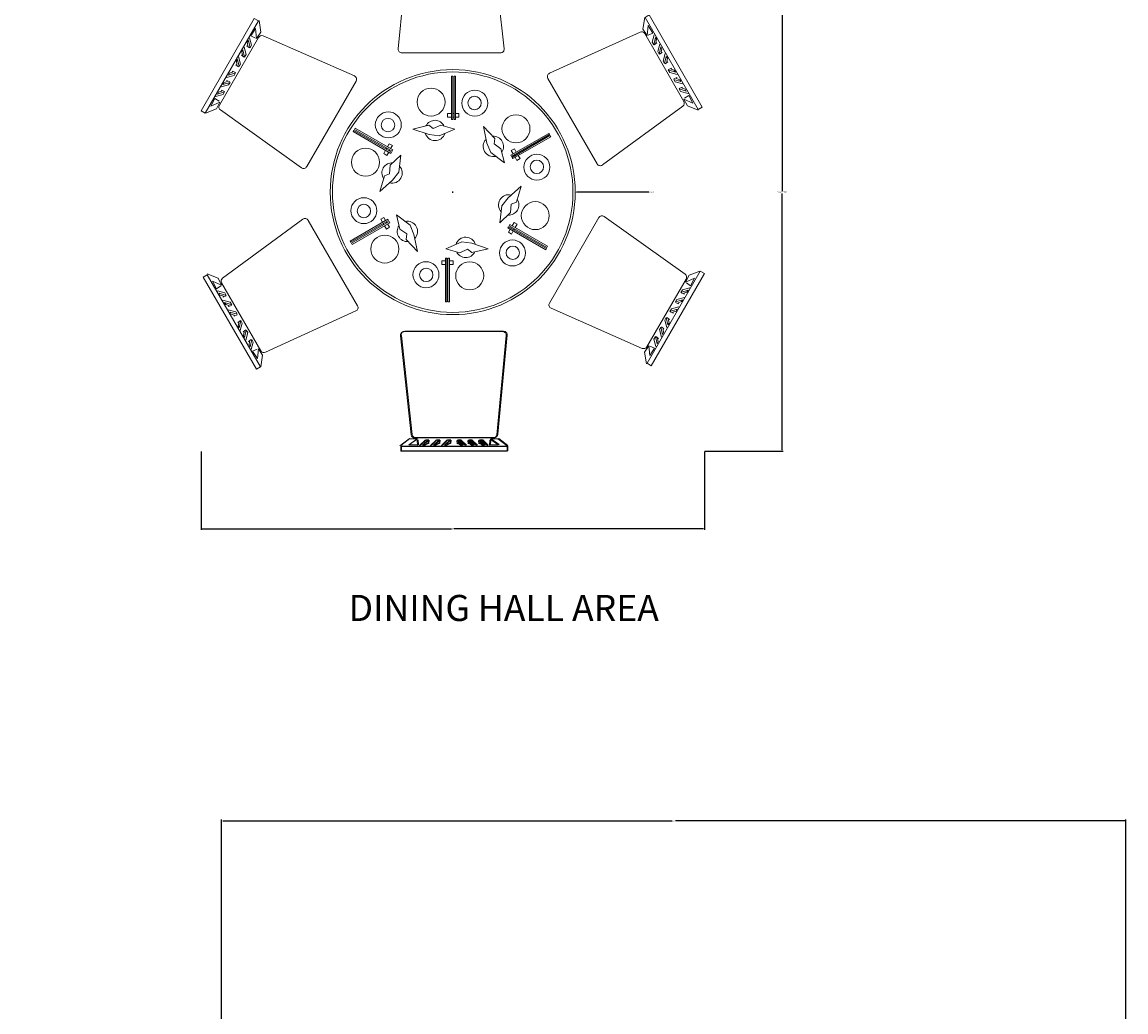
# Model space of a CAD drawing. Units: inches. Extents: x 1865 to 2541, y 1997 to 2759.
# Tile 4 of 11: x 2155 to 2346, y 2234 to 2405. Entities that reach past the tile are written whole.
import ezdxf

# ---------------------------------------------------------------- set-up
doc = ezdxf.new("R2010")
doc.units = ezdxf.units.IN
for name, color, linetype, lineweight in [('A-ANNO-DIMS', 2, 'Continuous', 18), ('A-AREA-IDEN', 4, 'Continuous', 18), ('DINING TABLE', 120, 'Continuous', 13)]:
    doc.layers.add(name, color=color, linetype=linetype, lineweight=lineweight)
doc.styles.get("Standard").update_dxf_attribs({"font": 'arial.ttf'})
doc.dimstyles.get("Standard").update_dxf_attribs({"dimtxt": 0.18, "dimasz": 0.18, "dimexe": 0.18, "dimexo": 0.0625, "dimgap": 0.09, "dimtad": 0, "dimtih": 1, "dimtoh": 1, "dimdec": 4, "dimzin": 0, "dimdsep": 46, "dimtxsty": 'Standard', "dimcen": 0.09, "dimadec": 0, "dimazin": 0, "dimtfac": 1, "dimtdec": 4, "dimtofl": 0, "dimtmove": 0, "dimatfit": 3, "dimfxl": 1, "dimtolj": 1, "dimtzin": 0, "dimarcsym": 0})

# ---------------------------------------------------------------- blocks, each defined once
blk = doc.blocks.new('A$C45501D90')
for p, q in [((-242.2, 1133.5), (224, 1133.5)), ((-242.2, 1112.8), (-242.2, 1133.5)), ((224, 1112.8), (-242.2, 1112.8)), ((224, 1112.8), (187.3, 1079.2)), ((224, 1133.5), (224, 1112.8)), ((-242.2, 1111.2), (-202.3, 1079.2)), ((-203.9, 1106.4), (-165.6, 1108)), ((-168.8, 1080.8), (-203.9, 1106.4)), ((-202.3, 1079.2), (-168.8, 1080.8)), ((161.8, 1076.1), (-181.4, 1076.1)), ((-165.6, 1108), (-167.2, 1085.6)), ((-156, 1109.6), (-132, 1085.6)), ((-119.3, 1085.6), (-143.2, 1108)), ((-143.2, 1108), (-133.6, 1108)), ((-133.6, 1108), (-122.5, 1098.4)), ((-132, 1085.6), (-119.3, 1085.6)), ((-122.5, 1098.4), (-119.3, 1101.6)), ((-119.3, 1101.6), (-117.7, 1087.2)), ((-108.1, 1109.6), (-84.1, 1085.6)), ((-71.4, 1085.6), (-95.3, 1108)), ((-95.3, 1108), (-85.7, 1108)), ((-85.7, 1108), (-74.6, 1098.4)), ((-84.1, 1085.6), (-71.4, 1085.6)), ((-74.6, 1098.4), (-71.4, 1101.6)), ((-71.4, 1101.6), (-69.8, 1087.2)), ((-60.2, 1109.6), (-36.2, 1085.6)), ((-23.5, 1085.6), (-47.4, 1108)), ((-47.4, 1108), (-37.8, 1108)), ((-37.8, 1108), (-26.7, 1098.4)), ((-36.2, 1085.6), (-23.5, 1085.6)), ((-26.7, 1098.4), (-23.5, 1101.6)), ((-23.5, 1101.6), (-21.9, 1087.2)), ((8.5, 1101.6), (6.9, 1087.2)), ((8.5, 1085.6), (32.4, 1108)), ((11.6, 1098.4), (8.5, 1101.6)), ((21.2, 1085.6), (8.5, 1085.6)), ((22.8, 1108), (11.6, 1098.4)), ((45.2, 1109.6), (21.2, 1085.6)), ((32.4, 1108), (22.8, 1108)), ((56.3, 1101.6), (54.8, 1087.2)), ((56.3, 1085.6), (80.3, 1108)), ((59.5, 1098.4), (56.3, 1101.6)), ((69.1, 1085.6), (56.3, 1085.6)), ((70.7, 1108), (59.5, 1098.4)), ((93.1, 1109.6), (69.1, 1085.6)), ((80.3, 1108), (70.7, 1108)), ((104.2, 1101.6), (102.6, 1087.2)), ((104.2, 1085.6), (128.2, 1108)), ((107.4, 1098.4), (104.2, 1101.6)), ((117, 1085.6), (104.2, 1085.6)), ((118.6, 1108), (107.4, 1098.4)), ((141, 1109.6), (117, 1085.6)), ((128.2, 1108), (118.6, 1108)), ((188.9, 1106.4), (150.5, 1108)), ((150.5, 1108), (152.1, 1085.6)), ((153.7, 1080.8), (188.9, 1106.4)), ((187.3, 1079.2), (153.7, 1080.8)), ((-197.3, 1061.6), (-238.9, 627.6)), ((225.2, 627.8), (177.6, 1061.8)), ((842.6, 766.1), (860.5, 776.5)), ((860.5, 776.5), (1093.6, 372.8)), ((-1102.7, 357), (-869.7, 760.7)), ((-851.7, 750.4), (-1084.8, 346.6)), ((-869.7, 760.7), (-851.7, 750.4)), ((-848.7, 752.3), (-841, 701.8)), ((841.2, 765.3), (833.5, 714.8)), ((1075.7, 362.4), (842.6, 766.1)), ((851.7, 686.6), (856.2, 729.8)), ((856.2, 729.8), (876.7, 697.4)), ((-851, 678.1), (-1022.6, 380.9)), ((-863.7, 716.7), (-884.3, 684.4)), ((-884.3, 684.4), (-864.1, 674.6)), ((-859.2, 673.6), (-863.7, 716.7)), ((-841, 701.8), (-859.2, 673.6)), ((-431.1, 509), (-830.8, 684.8)), ((820.7, 701.7), (424.1, 520.7)), ((833.5, 714.8), (851.7, 686.6)), ((1012.8, 397.9), (841.2, 695.1)), ((876.7, 697.4), (856.6, 687.6)), ((882.9, 689.9), (874.2, 657.2)), ((880.6, 646.1), (887.9, 678)), ((887.9, 678), (892.7, 669.7)), ((-914.4, 635.4), (-905.6, 602.7)), ((-897.5, 642.2), (-901.9, 641.1)), ((-901.9, 641.1), (-890.2, 632.5)), ((-895.4, 665), (-900.2, 656.7)), ((-900.2, 656.7), (-897.5, 642.2)), ((-888.1, 633.1), (-895.4, 665)), ((-890.4, 676.9), (-881.7, 644.2)), ((-881.7, 644.2), (-888.1, 633.1)), ((874.2, 657.2), (880.6, 646.1)), ((894.4, 654.1), (882.7, 645.5)), ((892.7, 669.7), (890, 655.2)), ((890, 655.2), (894.4, 654.1)), ((906.9, 648.4), (898.1, 615.7)), ((904.5, 604.6), (911.9, 636.5)), ((911.9, 636.5), (916.7, 628.2)), ((-943.3, 582), (-948.1, 573.8)), ((-936, 550.1), (-943.3, 582)), ((-938.3, 593.9), (-929.6, 561.2)), ((-921.5, 600.8), (-925.8, 599.6)), ((-925.8, 599.6), (-914.2, 591)), ((-919.4, 623.5), (-924.2, 615.2)), ((-924.2, 615.2), (-921.5, 600.8)), ((-912, 591.6), (-919.4, 623.5)), ((-905.6, 602.7), (-912, 591.6)), ((-223, 610.1), (209.4, 610.1)), ((898.1, 615.7), (904.5, 604.6)), ((918.3, 612.6), (906.7, 604)), ((916.7, 628.2), (914, 613.8)), ((914, 613.8), (918.3, 612.6)), ((930.8, 606.9), (922.1, 574.2)), ((928.4, 563.1), (935.8, 595.1)), ((935.8, 595.1), (940.6, 586.8)), ((940.6, 586.8), (937.9, 572.3)), ((-945.4, 559.3), (-949.8, 558.1)), ((-949.8, 558.1), (-938.1, 549.6)), ((-948.1, 573.8), (-945.4, 559.3)), ((-929.6, 561.2), (-936, 550.1)), ((922.1, 574.2), (928.4, 563.1)), ((942.3, 571.1), (930.6, 562.6)), ((937.9, 572.3), (942.3, 571.1)), ((950.8, 524.4), (944.4, 535.5)), ((944.4, 535.5), (975.7, 525.9)), ((958.2, 543.5), (945, 537.7)), ((957.1, 539.1), (958.2, 543.5)), ((970.9, 534.2), (957.1, 539.1)), ((975.7, 525.9), (970.9, 534.2)), ((-1002.4, 479.7), (-988.5, 484.6)), ((-991, 502.7), (-958.3, 511.4)), ((-988.5, 484.6), (-989.7, 489)), ((-989.7, 489), (-976.5, 483.2)), ((-951.9, 522.5), (-983.2, 512.9)), ((-983.2, 512.9), (-978.5, 521.2)), ((-978.5, 521.2), (-964.6, 526.1)), ((-964.6, 526.1), (-965.7, 530.5)), ((-965.7, 530.5), (-952.5, 524.7)), ((-958.3, 511.4), (-951.9, 522.5)), ((-639.9, 111.9), (-423.7, 486.4)), ((-5.6, 508.7, 90.8), (0.4, 508.7, 90.8)), ((-5.6, 317.7, 90.8), (-5.6, 508.7, 90.8)), ((0.4, 508.7, 90.8), (0.4, 317.7, 90.8)), ((5.8, 317.7, 90.8), (5.8, 508.7, 90.8)), ((5.8, 508.7, 90.8), (11.8, 508.7, 90.8)), ((11.8, 508.7, 90.8), (11.8, 317.7, 90.8)), ((416.9, 498.2), (633.1, 123.7)), ((983.5, 515.7), (950.8, 524.4)), ((968.4, 494), (999.7, 484.4)), ((974.7, 483), (968.4, 494)), ((982.2, 502), (968.9, 496.2)), ((981, 497.6), (982.2, 502)), ((994.9, 492.7), (981, 497.6)), ((999.7, 484.4), (994.9, 492.7)), ((-999.8, 439.5), (-1031.1, 430)), ((-1031.1, 430), (-1026.3, 438.3)), ((-1026.3, 438.3), (-1012.5, 443.1)), ((-1015, 461.2), (-982.3, 469.9)), ((-1012.5, 443.1), (-1013.6, 447.5)), ((-1013.6, 447.5), (-1000.4, 441.7)), ((-975.9, 481), (-1007.2, 471.4)), ((-1007.2, 471.4), (-1002.4, 479.7)), ((-1006.2, 428.5), (-999.8, 439.5)), ((-982.3, 469.9), (-975.9, 481)), ((1007.4, 474.2), (974.7, 483)), ((998.7, 441.5), (992.3, 452.5)), ((992.3, 452.5), (1023.6, 443)), ((1006.1, 460.5), (992.9, 454.7)), ((1031.4, 432.7), (998.7, 441.5)), ((1005, 456.2), (1006.1, 460.5)), ((1018.8, 451.3), (1005, 456.2)), ((1023.6, 443), (1018.8, 451.3)), ((-1060.1, 376.6), (-1042.3, 410.6)), ((-1020.4, 394.3), (-1060.1, 376.6)), ((-1042.3, 410.6), (-1023.8, 398.1)), ((-1038.9, 419.7), (-1006.2, 428.5)), ((-1035.8, 364.4), (-1020.4, 394.3)), ((1028.3, 377.5), (1012.9, 407.3)), ((1012.9, 407.3), (1052.6, 389.6)), ((1034.8, 423.6), (1016.3, 411.1)), ((1052.6, 389.6), (1034.8, 423.6)), ((-1084.8, 346.6), (-1102.7, 357)), ((-1083.4, 345.8), (-1035.8, 364.4)), ((-1018, 360), (-663, 106.9)), ((-22.3, 329.1, 90.8), (-22.3, 344.6, 90.8)), ((-22.3, 344.6, 90.8), (-5.6, 344.6, 90.8)), ((0.4, 344.6, 90.8), (5.8, 344.6, 90.8)), ((11.8, 344.6, 90.8), (27.3, 344.6, 90.8)), ((27.3, 344.6, 90.8), (27.3, 329.1, 90.8)), ((656.3, 118.9), (1008.4, 377.1)), ((1075.9, 358.8), (1028.3, 377.5)), ((1093.6, 372.8), (1075.7, 362.4)), ((-175.3, 276.1, 90.8), (-104.8, 293.2, 90.8)), ((-104.8, 293.2, 90.8), (-85.5, 278.4, 90.8)), ((-85.5, 278.4, 90.8), (-52.1, 293.9, 90.8)), ((-52.1, 293.9, 90.8), (9.5, 276.1, 90.8)), ((-5.6, 329.1, 90.8), (-22.3, 329.1, 90.8)), ((0.4, 317.7, 90.8), (-5.6, 317.7, 90.8)), ((5.8, 329.1, 90.8), (0.4, 329.1, 90.8)), ((11.8, 317.7, 90.8), (5.8, 317.7, 90.8)), ((27.3, 329.1, 90.8), (11.8, 329.1, 90.8)), ((-436.3, 265.3, 90.8), (-433.3, 270.5, 90.8)), ((-270.9, 169.9, 90.8), (-436.3, 265.3, 90.8)), ((-433.3, 270.5, 90.8), (-267.9, 175, 90.8)), ((-430.6, 275.2, 90.8), (-427.6, 280.3, 90.8)), ((-265.2, 179.7, 90.8), (-430.6, 275.2, 90.8)), ((-427.6, 280.3, 90.8), (-262.3, 184.9, 90.8)), ((-103.3, 252.4, 90.8), (-175.3, 276.1, 90.8)), ((-59.5, 246.5, 90.8), (-103.3, 252.4, 90.8)), ((9.5, 276.1, 90.8), (-59.5, 246.5, 90.8)), ((134.3, 288, 90.8), (184.3, 235.5, 90.8)), ((149.7, 213.9, 90.8), (134.3, 288, 90.8)), ((255.2, 161.9, 90.8), (420.6, 257.3, 90.8)), ((423.5, 252.2, 90.8), (258.2, 156.7, 90.8)), ((260.9, 152, 90.8), (426.2, 247.5, 90.8)), ((429.2, 242.3, 90.8), (263.8, 146.9, 90.8)), ((420.6, 257.3, 90.8), (423.5, 252.2, 90.8)), ((426.2, 247.5, 90.8), (429.2, 242.3, 90.8)), ((-285.5, 198.3, 90.8), (-277.8, 211.7, 90.8)), ((-277.8, 211.7, 90.8), (-264.3, 204, 90.8)), ((-264.3, 204, 90.8), (-272.1, 190.5, 90.8)), ((166.5, 173, 90.8), (149.7, 213.9, 90.8)), ((184.3, 235.5, 90.8), (181.1, 211.4, 90.8)), ((181.1, 211.4, 90.8), (211.3, 190.3, 90.8)), ((-302.5, 168.8, 90.8), (-294.2, 183.3, 90.8)), ((-289.1, 161.1, 90.8), (-302.5, 168.8, 90.8)), ((-291.2, 188.5, 90.8), (-288.5, 193.1, 90.8)), ((-280.7, 175.5, 90.8), (-289.1, 161.1, 90.8)), ((-275.1, 185.4, 90.8), (-277.8, 180.7, 90.8)), ((-273.6, 117.6, 90.8), (-227.4, 162.1, 90.8)), ((-267.9, 175, 90.8), (-270.9, 169.9, 90.8)), ((-262.3, 184.9, 90.8), (-265.2, 179.7, 90.8)), ((-227.4, 162.1, 90.8), (-236.2, 87.5, 90.8)), ((226.7, 128.1, 90.8), (166.5, 173, 90.8)), ((211.3, 190.3, 90.8), (226.7, 128.1, 90.8)), ((258.2, 156.7, 90.8), (255.2, 161.9, 90.8)), ((256.6, 182, 90.8), (270.1, 189.8, 90.8)), ((265, 167.5, 90.8), (256.6, 182, 90.8)), ((263.8, 146.9, 90.8), (260.9, 152, 90.8)), ((270.7, 157.7, 90.8), (268, 162.4, 90.8)), ((270.1, 189.8, 90.8), (278.4, 175.3, 90.8)), ((281.4, 139.1, 90.8), (273.7, 152.5, 90.8)), ((281.4, 170.1, 90.8), (284.1, 165.5, 90.8)), ((294.9, 146.8, 90.8), (281.4, 139.1, 90.8)), ((287.1, 160.3, 90.8), (294.9, 146.8, 90.8)), ((-276.8, 80.9, 90.8), (-273.6, 117.6, 90.8)), ((-319.8, 2.1, 90.8), (-299.3, 71.7, 90.8)), ((-263.2, 52.5, 90.8), (-319.8, 2.1, 90.8)), ((-299.3, 71.7, 90.8), (-276.8, 80.9, 90.8)), ((-236.2, 87.5, 90.8), (-263.2, 52.5, 90.8)), ((242.9, -24.6, 90.8), (299.4, 25.9, 90.8)), ((299.4, 25.9, 90.8), (278.9, -43.7, 90.8)), ((215.8, -59.5, 90.8), (242.9, -24.6, 90.8)), ((278.9, -43.7, 90.8), (256.4, -53, 90.8)), ((207, -134.1, 90.8), (215.8, -59.5, 90.8)), ((253.2, -89.7, 90.8), (207, -134.1, 90.8)), ((256.4, -53, 90.8), (253.2, -89.7, 90.8)), ((-656.3, -118.9), (-1008.4, -377.1)), ((-416.9, -498.2), (-633.1, -123.7)), ((-449.6, -214.4, 90.8), (-284.2, -118.9, 90.8)), ((-281.2, -124.1, 90.8), (-446.6, -219.5, 90.8)), ((-443.9, -224.2, 90.8), (-278.5, -128.7, 90.8)), ((-275.5, -133.9, 90.8), (-440.9, -229.4, 90.8)), ((-315.2, -118.9, 90.8), (-301.8, -111.1, 90.8)), ((-307.5, -132.3, 90.8), (-315.2, -118.9, 90.8)), ((-301.8, -142.1, 90.8), (-304.5, -137.5, 90.8)), ((-301.8, -111.1, 90.8), (-294, -124.6, 90.8)), ((-291, -129.7, 90.8), (-288.3, -134.4, 90.8)), ((-285.4, -139.5, 90.8), (-277, -154, 90.8)), ((-284.2, -118.9, 90.8), (-281.2, -124.1, 90.8)), ((-278.5, -128.7, 90.8), (-275.5, -133.9, 90.8)), ((-247, -100.1, 90.8), (-186.8, -145, 90.8)), ((-231.7, -162.3, 90.8), (-247, -100.1, 90.8)), ((-186.8, -145, 90.8), (-170.1, -185.9, 90.8)), ((247.6, -147.1, 90.8), (250.6, -141.9, 90.8)), ((250.6, -141.9, 90.8), (415.9, -237.4, 90.8)), ((260.4, -147.6, 90.8), (268.7, -133.1, 90.8)), ((268.7, -133.1, 90.8), (282.2, -140.8, 90.8)), ((282.2, -140.8, 90.8), (273.8, -155.3, 90.8)), ((639.9, -111.9), (423.7, -486.4)), ((1018, -360), (663, -106.9)), ((-290.4, -161.8, 90.8), (-298.8, -147.3, 90.8)), ((-277, -154, 90.8), (-290.4, -161.8, 90.8)), ((-201.5, -183.4, 90.8), (-231.7, -162.3, 90.8)), ((-204.7, -207.6, 90.8), (-201.5, -183.4, 90.8)), ((-170.1, -185.9, 90.8), (-154.7, -260.1, 90.8)), ((241.9, -156.9, 90.8), (244.9, -151.7, 90.8)), ((407.3, -252.4, 90.8), (241.9, -156.9, 90.8)), ((244, -176, 90.8), (251.7, -162.5, 90.8)), ((257.4, -183.7, 90.8), (244, -176, 90.8)), ((244.9, -151.7, 90.8), (410.3, -247.2, 90.8)), ((413, -242.5, 90.8), (247.6, -147.1, 90.8)), ((254.7, -157.4, 90.8), (257.4, -152.7, 90.8)), ((265.2, -170.3, 90.8), (257.4, -183.7, 90.8)), ((270.8, -160.5, 90.8), (268.1, -165.1, 90.8)), ((-446.6, -219.5, 90.8), (-449.6, -214.4, 90.8)), ((-440.9, -229.4, 90.8), (-443.9, -224.2, 90.8)), ((-154.7, -260.1, 90.8), (-204.7, -207.6, 90.8)), ((-29.8, -248.2, 90.8), (39.2, -218.5, 90.8)), ((39.2, -218.5, 90.8), (83, -224.4, 90.8)), ((83, -224.4, 90.8), (154.9, -248.2, 90.8)), ((415.9, -237.4, 90.8), (413, -242.5, 90.8)), ((-32.1, -480.7, 90.8), (-32.1, -289.8, 90.8)), ((-32.1, -289.8, 90.8), (-26.1, -289.8, 90.8)), ((31.8, -266, 90.8), (-29.8, -248.2, 90.8)), ((-26.1, -289.8, 90.8), (-26.1, -480.7, 90.8)), ((-20.8, -480.7, 90.8), (-20.8, -289.8, 90.8)), ((-20.8, -289.8, 90.8), (-14.8, -289.8, 90.8)), ((-14.8, -289.8, 90.8), (-14.8, -480.7, 90.8)), ((65.2, -250.4, 90.8), (31.8, -266, 90.8)), ((84.4, -265.2, 90.8), (65.2, -250.4, 90.8)), ((154.9, -248.2, 90.8), (84.4, -265.2, 90.8)), ((410.3, -247.2, 90.8), (407.3, -252.4, 90.8)), ((-47.6, -316.6, 90.8), (-47.6, -301.1, 90.8)), ((-47.6, -301.1, 90.8), (-32.1, -301.1, 90.8)), ((-32.1, -316.6, 90.8), (-47.6, -316.6, 90.8)), ((-26.1, -301.1, 90.8), (-20.8, -301.1, 90.8)), ((-20.8, -316.6, 90.8), (-26.1, -316.6, 90.8)), ((-14.8, -301.1, 90.8), (1.9, -301.1, 90.8)), ((1.9, -316.6, 90.8), (-14.8, -316.6, 90.8)), ((1.9, -301.1, 90.8), (1.9, -316.6, 90.8)), ((-1093.6, -372.8), (-1075.7, -362.4)), ((-860.5, -776.5), (-1093.6, -372.8)), ((-1075.9, -358.8), (-1028.3, -377.5)), ((-1075.7, -362.4), (-842.6, -766.1)), ((-1028.3, -377.5), (-1012.9, -407.3)), ((851, -678.1), (1022.6, -380.9)), ((851.7, -750.4), (1084.8, -346.6)), ((1102.7, -357), (869.7, -760.7)), ((1035.8, -364.4), (1020.4, -394.3)), ((1020.4, -394.3), (1060.1, -376.6)), ((1083.4, -345.8), (1035.8, -364.4)), ((1060.1, -376.6), (1042.3, -410.6)), ((1084.8, -346.6), (1102.7, -357)), ((-1052.6, -389.6), (-1034.8, -423.6)), ((-1012.9, -407.3), (-1052.6, -389.6)), ((-1034.8, -423.6), (-1016.3, -411.1)), ((-1031.4, -432.7), (-998.7, -441.5)), ((-1012.8, -397.9), (-841.2, -695.1)), ((1006.2, -428.5), (999.8, -439.5)), ((999.8, -439.5), (1031.1, -430)), ((1038.9, -419.7), (1006.2, -428.5)), ((1042.3, -410.6), (1023.8, -398.1)), ((1031.1, -430), (1026.3, -438.3)), ((-1023.6, -443), (-1018.8, -451.3)), ((-992.3, -452.5), (-1023.6, -443)), ((-1018.8, -451.3), (-1005, -456.2)), ((-1007.4, -474.2), (-974.7, -483)), ((-1006.1, -460.5), (-992.9, -454.7)), ((-1005, -456.2), (-1006.1, -460.5)), ((-998.7, -441.5), (-992.3, -452.5)), ((-974.7, -483), (-968.4, -494)), ((-26.1, -480.7, 90.8), (-32.1, -480.7, 90.8)), ((-14.8, -480.7, 90.8), (-20.8, -480.7, 90.8)), ((982.3, -469.9), (975.9, -481)), ((975.9, -481), (1007.2, -471.4)), ((989.7, -489), (976.5, -483.2)), ((1015, -461.2), (982.3, -469.9)), ((1002.4, -479.7), (988.5, -484.6)), ((1013.6, -447.5), (1000.4, -441.7)), ((1007.2, -471.4), (1002.4, -479.7)), ((1026.3, -438.3), (1012.5, -443.1)), ((1012.5, -443.1), (1013.6, -447.5)), ((-968.4, -494), (-999.7, -484.4)), ((-999.7, -484.4), (-994.9, -492.7)), ((-994.9, -492.7), (-981, -497.6)), ((-983.5, -515.7), (-950.8, -524.4)), ((-982.2, -502), (-968.9, -496.2)), ((-981, -497.6), (-982.2, -502)), ((-944.4, -535.5), (-975.7, -525.9)), ((-975.7, -525.9), (-970.9, -534.2)), ((-950.8, -524.4), (-944.4, -535.5)), ((-820.7, -701.7), (-424.1, -520.7)), ((431.1, -509), (830.8, -684.8)), ((958.3, -511.4), (951.9, -522.5)), ((951.9, -522.5), (983.2, -512.9)), ((965.7, -530.5), (952.5, -524.7)), ((991, -502.7), (958.3, -511.4)), ((978.5, -521.2), (964.6, -526.1)), ((964.6, -526.1), (965.7, -530.5)), ((983.2, -512.9), (978.5, -521.2)), ((988.5, -484.6), (989.7, -489)), ((-970.9, -534.2), (-957.1, -539.1)), ((-958.2, -543.5), (-945, -537.7)), ((-957.1, -539.1), (-958.2, -543.5)), ((-942.3, -571.1), (-930.6, -562.6)), ((-937.9, -572.3), (-942.3, -571.1)), ((-940.6, -586.8), (-937.9, -572.3)), ((-928.4, -563.1), (-935.8, -595.1)), ((-930.8, -606.9), (-922.1, -574.2)), ((-922.1, -574.2), (-928.4, -563.1)), ((929.6, -561.2), (936, -550.1)), ((938.3, -593.9), (929.6, -561.2)), ((936, -550.1), (943.3, -582)), ((949.8, -558.1), (938.1, -549.6)), ((943.3, -582), (948.1, -573.8)), ((945.4, -559.3), (949.8, -558.1)), ((948.1, -573.8), (945.4, -559.3)), ((-935.8, -595.1), (-940.6, -586.8)), ((-918.3, -612.6), (-906.7, -604)), ((-914, -613.8), (-918.3, -612.6)), ((-916.7, -628.2), (-914, -613.8)), ((-911.9, -636.5), (-916.7, -628.2)), ((-904.5, -604.6), (-911.9, -636.5)), ((-906.9, -648.4), (-898.1, -615.7)), ((-898.1, -615.7), (-904.5, -604.6)), ((-225.2, -627.8), (-177.6, -1061.8)), ((218.9, -611.6), (-213.5, -611.6)), ((223, -610.1), (-209.4, -610.1)), ((197.3, -1061.6), (238.9, -627.6)), ((905.6, -602.7), (912, -591.6)), ((914.4, -635.4), (905.6, -602.7)), ((912, -591.6), (919.4, -623.5)), ((925.8, -599.6), (914.2, -591)), ((919.4, -623.5), (924.2, -615.2)), ((921.5, -600.8), (925.8, -599.6)), ((924.2, -615.2), (921.5, -600.8)), ((-894.4, -654.1), (-882.7, -645.5)), ((-890, -655.2), (-894.4, -654.1)), ((-892.7, -669.7), (-890, -655.2)), ((-887.9, -678), (-892.7, -669.7)), ((-880.6, -646.1), (-887.9, -678)), ((-882.9, -689.9), (-874.2, -657.2)), ((-874.2, -657.2), (-880.6, -646.1)), ((-229.3, -629.3), (-181.8, -1063.3)), ((193.2, -1063.1), (234.8, -629.1)), ((841, -701.8), (859.2, -673.6)), ((859.2, -673.6), (863.7, -716.7)), ((884.3, -684.4), (864.1, -674.6)), ((881.7, -644.2), (888.1, -633.1)), ((890.4, -676.9), (881.7, -644.2)), ((888.1, -633.1), (895.4, -665)), ((901.9, -641.1), (890.2, -632.5)), ((895.4, -665), (900.2, -656.7)), ((897.5, -642.2), (901.9, -641.1)), ((900.2, -656.7), (897.5, -642.2)), ((-876.7, -697.4), (-856.6, -687.6)), ((-856.2, -729.8), (-876.7, -697.4)), ((-851.7, -686.6), (-856.2, -729.8)), ((-833.5, -714.8), (-851.7, -686.6)), ((-841.2, -765.3), (-833.5, -714.8)), ((848.7, -752.3), (841, -701.8)), ((863.7, -716.7), (884.3, -684.4)), ((-842.6, -766.1), (-860.5, -776.5)), ((869.7, -760.7), (851.7, -750.4)), ((-231.3, -1112.7), (-191.4, -1080.8)), ((-227.2, -1111.2), (-187.3, -1079.2)), ((-157.9, -1082.4), (-193, -1107.9)), ((-193, -1107.9), (-154.7, -1109.5)), ((-191.4, -1080.8), (-157.9, -1082.4)), ((-153.7, -1080.8), (-188.9, -1106.4)), ((-188.9, -1106.4), (-150.5, -1108)), ((-187.3, -1079.2), (-153.7, -1080.8)), ((-165.9, -1077.6), (177.3, -1077.6)), ((-161.8, -1076.1), (181.4, -1076.1)), ((-154.7, -1109.5), (-156.3, -1087.1)), ((-150.5, -1108), (-152.1, -1085.6)), ((-145.1, -1111.1), (-121.1, -1087.1)), ((-141, -1109.6), (-117, -1085.6)), ((-108.4, -1087.1), (-132.3, -1109.5)), ((-132.3, -1109.5), (-122.7, -1109.5)), ((-104.2, -1085.6), (-128.2, -1108)), ((-128.2, -1108), (-118.6, -1108)), ((-122.7, -1109.5), (-111.6, -1099.9)), ((-121.1, -1087.1), (-108.4, -1087.1)), ((-118.6, -1108), (-107.4, -1098.4)), ((-117, -1085.6), (-104.2, -1085.6)), ((-111.6, -1099.9), (-108.4, -1103.1)), ((-108.4, -1103.1), (-106.8, -1088.7)), ((-107.4, -1098.4), (-104.2, -1101.6)), ((-104.2, -1101.6), (-102.6, -1087.2)), ((-97.2, -1111.1), (-73.2, -1087.1)), ((-93.1, -1109.6), (-69.1, -1085.6)), ((-60.5, -1087.1), (-84.4, -1109.5)), ((-84.4, -1109.5), (-74.8, -1109.5)), ((-56.3, -1085.6), (-80.3, -1108)), ((-80.3, -1108), (-70.7, -1108)), ((-74.8, -1109.5), (-63.7, -1099.9)), ((-73.2, -1087.1), (-60.5, -1087.1)), ((-70.7, -1108), (-59.5, -1098.4)), ((-69.1, -1085.6), (-56.3, -1085.6)), ((-63.7, -1099.9), (-60.5, -1103.1)), ((-60.5, -1103.1), (-58.9, -1088.7)), ((-59.5, -1098.4), (-56.3, -1101.6)), ((-56.3, -1101.6), (-54.8, -1087.2)), ((-49.3, -1111.1), (-25.3, -1087.1)), ((-45.2, -1109.6), (-21.2, -1085.6)), ((-12.6, -1087.1), (-36.5, -1109.5)), ((-36.5, -1109.5), (-26.9, -1109.5)), ((-8.5, -1085.6), (-32.4, -1108)), ((-32.4, -1108), (-22.8, -1108)), ((-26.9, -1109.5), (-15.8, -1099.9)), ((-25.3, -1087.1), (-12.6, -1087.1)), ((-22.8, -1108), (-11.6, -1098.4)), ((-21.2, -1085.6), (-8.5, -1085.6)), ((-15.8, -1099.9), (-12.6, -1103.1)), ((-12.6, -1103.1), (-11, -1088.7)), ((-11.6, -1098.4), (-8.5, -1101.6)), ((-8.5, -1101.6), (-6.9, -1087.2)), ((19.4, -1103.1), (17.8, -1088.7)), ((19.4, -1087.1), (43.3, -1109.5)), ((32.1, -1087.1), (19.4, -1087.1)), ((22.6, -1099.9), (19.4, -1103.1)), ((23.5, -1101.6), (21.9, -1087.2)), ((33.7, -1109.5), (22.6, -1099.9)), ((23.5, -1085.6), (47.4, -1108)), ((36.2, -1085.6), (23.5, -1085.6)), ((26.7, -1098.4), (23.5, -1101.6)), ((37.8, -1108), (26.7, -1098.4)), ((56.1, -1111.1), (32.1, -1087.1)), ((43.3, -1109.5), (33.7, -1109.5)), ((60.2, -1109.6), (36.2, -1085.6)), ((47.4, -1108), (37.8, -1108)), ((67.3, -1103.1), (65.7, -1088.7)), ((67.3, -1087.1), (91.2, -1109.5)), ((80, -1087.1), (67.3, -1087.1)), ((70.4, -1099.9), (67.3, -1103.1)), ((71.4, -1101.6), (69.8, -1087.2)), ((81.6, -1109.5), (70.4, -1099.9)), ((71.4, -1085.6), (95.3, -1108)), ((84.1, -1085.6), (71.4, -1085.6)), ((74.6, -1098.4), (71.4, -1101.6)), ((85.7, -1108), (74.6, -1098.4)), ((104, -1111.1), (80, -1087.1)), ((91.2, -1109.5), (81.6, -1109.5)), ((108.1, -1109.6), (84.1, -1085.6)), ((95.3, -1108), (85.7, -1108)), ((115.1, -1103.1), (113.6, -1088.7)), ((115.1, -1087.1), (139.1, -1109.5)), ((127.9, -1087.1), (115.1, -1087.1)), ((118.3, -1099.9), (115.1, -1103.1)), ((119.3, -1101.6), (117.7, -1087.2)), ((129.5, -1109.5), (118.3, -1099.9)), ((119.3, -1085.6), (143.2, -1108)), ((132, -1085.6), (119.3, -1085.6)), ((122.5, -1098.4), (119.3, -1101.6)), ((133.6, -1108), (122.5, -1098.4)), ((151.9, -1111.1), (127.9, -1087.1)), ((139.1, -1109.5), (129.5, -1109.5)), ((156, -1109.6), (132, -1085.6)), ((143.2, -1108), (133.6, -1108)), ((161.4, -1109.5), (163, -1087.1)), ((199.8, -1107.9), (161.4, -1109.5)), ((198.2, -1080.8), (164.6, -1082.4)), ((164.6, -1082.4), (199.8, -1107.9)), ((165.6, -1108), (167.2, -1085.6)), ((203.9, -1106.4), (165.6, -1108)), ((202.3, -1079.2), (168.8, -1080.8)), ((168.8, -1080.8), (203.9, -1106.4)), ((238.1, -1112.7), (198.2, -1080.8)), ((242.2, -1111.2), (202.3, -1079.2)), ((-228.1, -1114.3), (238.1, -1114.3)), ((-228.1, -1135), (-228.1, -1114.3)), ((238.1, -1135), (-228.1, -1135)), ((-224, -1112.8), (242.2, -1112.8)), ((-224, -1133.5), (-224, -1112.8)), ((242.2, -1133.5), (-224, -1133.5)), ((238.1, -1114.3), (238.1, -1135)), ((242.2, -1112.8), (242.2, -1133.5))]:
    blk.add_line(p, q)
for centre, radius in [((0, 0), 537), ((0, 0), 527), ((-94.8, 394.7, 90.8), 61.3), ((96.9, 390, 90.8), 56.9), ((95.5, 390.7, 90.8), 29.4), ((-282.3, 294.7, 90.8), 56.9), ((277.2, 277.6, 90.8), 61.3), ((-283.5, 293.9, 90.8), 29.4), ((-382.1, 131.1, 90.8), 61.3), ((369, 109.3, 90.8), 56.9), ((368.9, 110.8, 90.8), 29.4), ((-389.3, -81.3, 90.8), 56.9), ((361.8, -103.1, 90.8), 61.3), ((-389.2, -82.8, 90.8), 29.4), ((-297.5, -249.6, 90.8), 61.3), ((261.9, -266.7, 90.8), 56.9), ((263.2, -265.9, 90.8), 29.4), ((-117.2, -362, 90.8), 56.9), ((-115.9, -362.7, 90.8), 29.4), ((74.4, -366.7, 90.8), 61.3)]:
    blk.add_circle(centre, radius)
for centre, radius, start, end in [((-181.4, 1060.1), 16, 90, 174.5199), ((161.8, 1060.1), 16, 6.2572, 90), ((-837.2, 670.1), 16, 66.2572, 150), ((827.4, 687.1), 16, 30, 114.5199), ((-223, 626.1), 16, 174.5199, 270), ((209.4, 626.1), 16, 270, 6.2572), ((-437.5, 494.4), 16, 330, 66.2572), ((430.7, 506.2), 16, 114.5199, 210), ((999, 389.9), 16, 306.2572, 30), ((-1008.8, 373), 16, 150, 234.5199), ((-77.3, 270.2, 90.8), 44.6, 25.8558, 153.3359), ((-77.3, 270.2, 90.8), 44.6, 195.9338, 342.9389), ((178.1, 200.3, 90.8), 44.6, 325.8558, 93.3359), ((178.1, 200.3, 90.8), 44.6, 135.9338, 282.9389), ((-653.7, 119.9), 16, 234.5199, 330), ((-265.7, 83.9, 90.8), 44.6, 85.8558, 213.3359), ((-265.7, 83.9, 90.8), 44.6, 255.9338, 42.9389), ((646.9, 131.7), 16, 210, 306.2572), ((245.3, -55.9, 90.8), 44.6, 75.9338, 222.9389), ((245.3, -55.9, 90.8), 44.6, 265.8558, 33.3359), ((-646.9, -131.7), 16, 30, 126.2572), ((-198.5, -172.3, 90.8), 44.6, 315.9338, 102.9389), ((653.7, -119.9), 16, 54.5199, 150), ((-198.5, -172.3, 90.8), 44.6, 145.8558, 273.3359), ((57, -242.2, 90.8), 44.6, 15.9338, 162.9389), ((57, -242.2, 90.8), 44.6, 205.8558, 333.3359), ((-999, -389.9), 16, 126.2572, 210), ((1008.8, -373), 16, 330, 54.5199), ((-430.7, -506.2), 16, 294.5199, 30), ((437.5, -494.4), 16, 150, 246.2572), ((-213.5, -627.6), 16, 90, 186.2572), ((-209.4, -626.1), 16, 90, 186.2572), ((218.9, -627.6), 16, 354.5199, 90), ((223, -626.1), 16, 354.5199, 90), ((-827.4, -687.1), 16, 210, 294.5199), ((837.2, -670.1), 16, 246.2572, 330), ((-165.9, -1061.6), 16, 186.2572, 270), ((-161.8, -1060.1), 16, 186.2572, 270), ((177.3, -1061.6), 16, 270, 354.5199), ((181.4, -1060.1), 16, 270, 354.5199)]:
    blk.add_arc(centre, radius, start, end)
blk = doc.blocks.new('*D38')
at = {"layer": 'A-ANNO-DIMS', "color": 0, "lineweight": -2, "transparency": 16777216}
for p, q in [((2273.08, 2420.54), (2286.59, 2420.54)), ((2286.41, 2420.36), (2286.41, 2376.07)), ((2286.41, 2331.41), (2286.41, 2375.7)), ((2273.08, 2331.23), (2286.59, 2331.23))]:
    blk.add_line(p, q, dxfattribs=at)
at = {"layer": 'A-ANNO-DIMS', "color": 0, "transparency": 16777216}
for points in [[(2286.38, 2420.36), (2286.44, 2420.36), (2286.41, 2420.54)], [(2286.38, 2331.41), (2286.44, 2331.41), (2286.41, 2331.23)]]:
    blk.add_solid(points, dxfattribs=at)
at = {"layer": 'Defpoints', "color": 0, "transparency": 16777216}
for p in [(2273.02, 2420.54), (2286.41, 2420.54), (2273.02, 2331.23)]:
    blk.add_point(p, dxfattribs=at)
at = {"layer": 'A-ANNO-DIMS', "color": 0, "transparency": 16777216, "insert": (2286.41, 2375.89), "char_height": 0.18, "attachment_point": 5}
blk.add_mtext('\\A1;DINING SET 89', dxfattribs=at)
blk = doc.blocks.new('*D39')
at = {"layer": 'A-ANNO-DIMS', "color": 0, "lineweight": -2, "transparency": 16777216}
for p, q in [((2186.19, 2331.17), (2186.19, 2317.65)), ((2273.02, 2331.17), (2273.02, 2317.65)), ((2186.37, 2317.83), (2229.38, 2317.83)), ((2272.84, 2317.83), (2229.82, 2317.83))]:
    blk.add_line(p, q, dxfattribs=at)
at = {"layer": 'A-ANNO-DIMS', "color": 0, "transparency": 16777216}
for points in [[(2186.37, 2317.86), (2186.37, 2317.8), (2186.19, 2317.83)], [(2272.84, 2317.86), (2272.84, 2317.8), (2273.02, 2317.83)]]:
    blk.add_solid(points, dxfattribs=at)
at = {"layer": 'Defpoints', "color": 0, "transparency": 16777216}
for p in [(2186.19, 2331.23), (2273.02, 2331.23), (2273.02, 2317.83)]:
    blk.add_point(p, dxfattribs=at)
at = {"layer": 'A-ANNO-DIMS', "color": 0, "transparency": 16777216, "insert": (2229.6, 2317.83), "char_height": 0.18, "attachment_point": 5}
blk.add_mtext('\\A1;87', dxfattribs=at)
blk = doc.blocks.new('*D41')
at = {"layer": 'A-ANNO-DIMS', "color": 0, "lineweight": -2, "transparency": 16777216}
for p, q in [((2503.31, 2721.45), (2540.92, 2721.45)), ((2540.74, 2721.27), (2540.74, 2378.49)), ((2540.74, 2035.35), (2540.74, 2378.13)), ((2136.19, 2035.17), (2540.92, 2035.17))]:
    blk.add_line(p, q, dxfattribs=at)
at = {"layer": 'A-ANNO-DIMS', "color": 0, "transparency": 16777216}
for points in [[(2540.71, 2721.27), (2540.77, 2721.27), (2540.74, 2721.45)], [(2540.71, 2035.35), (2540.77, 2035.35), (2540.74, 2035.17)]]:
    blk.add_solid(points, dxfattribs=at)
at = {"layer": 'Defpoints', "color": 0, "transparency": 16777216}
for p in [(2503.24, 2721.45), (2136.13, 2035.17), (2540.74, 2035.17)]:
    blk.add_point(p, dxfattribs=at)
at = {"layer": 'A-ANNO-DIMS', "color": 0, "transparency": 16777216, "insert": (2540.74, 2378.31), "char_height": 0.18, "attachment_point": 5}
blk.add_mtext('\\A1;686.3', dxfattribs=at)
blk = doc.blocks.new('*D54')
at = {"layer": 'A-ANNO-DIMS', "color": 0, "lineweight": -2, "transparency": 16777216}
for p, q in [((2189.74, 2230.01), (2189.74, 2267.63)), ((2189.92, 2267.45), (2267.46, 2267.45)), ((2345.56, 2267.45), (2268.02, 2267.45)), ((2345.74, 2230.01), (2345.74, 2267.63))]:
    blk.add_line(p, q, dxfattribs=at)
at = {"layer": 'A-ANNO-DIMS', "color": 0, "transparency": 16777216}
for points in [[(2189.92, 2267.48), (2189.92, 2267.42), (2189.74, 2267.45)], [(2345.56, 2267.48), (2345.56, 2267.42), (2345.74, 2267.45)]]:
    blk.add_solid(points, dxfattribs=at)
at = {"layer": 'Defpoints', "color": 0, "transparency": 16777216}
for p in [(2345.74, 2267.45), (2189.74, 2229.95), (2345.74, 2229.95)]:
    blk.add_point(p, dxfattribs=at)
at = {"layer": 'A-ANNO-DIMS', "color": 0, "transparency": 16777216, "insert": (2267.74, 2267.45), "char_height": 0.18, "attachment_point": 5}
blk.add_mtext('\\A1;156', dxfattribs=at)
blk = doc.blocks.new('*D84')
at = {"layer": 'A-ANNO-DIMS', "color": 0, "lineweight": -2, "transparency": 16777216}
for p, q in [((2229.51, 2375.91), (2229.69, 2375.91)), ((2229.6, 2375.82), (2229.6, 2376)), ((2263.43, 2375.91), (2250.93, 2375.91))]:
    blk.add_line(p, q, dxfattribs=at)
at = {"layer": 'A-ANNO-DIMS', "color": 0, "transparency": 16777216}
blk.add_solid([(2250.93, 2375.95), (2250.93, 2375.89), (2250.75, 2375.91)], dxfattribs=at)
at = {"layer": 'Defpoints', "color": 0, "transparency": 16777216}
for p in [(2208.46, 2375.91), (2250.75, 2375.91)]:
    blk.add_point(p, dxfattribs=at)
at = {"layer": 'A-ANNO-DIMS', "color": 0, "transparency": 16777216, "insert": (2263.99, 2375.91), "char_height": 0.18, "attachment_point": 5}
blk.add_mtext('\\A1;∅42.285', dxfattribs=at)

msp = doc.modelspace()

# ---------------------------------------------------------------- block references
at = {"layer": 'DINING TABLE', "xscale": 0.0393700787401575, "yscale": 0.0393700787401575, "zscale": 0.0393700787401575}
msp.add_blockref('A$C45501D90', (2229.6028, 2375.915, -3.5735), dxfattribs=at)

# ---------------------------------------------------------------- texts
at = {"layer": 'A-AREA-IDEN', "insert": (2211.6402, 2306.4059), "char_height": 4.5, "attachment_point": 1}
msp.add_mtext_dynamic_manual_height_columns('DINING HALL AREA', width=66.075761, gutter_width=12.5, heights=[0], dxfattribs=at)

# ---------------------------------------------------------------- dimensions: what is measured, and where the dimension line sits
at = {"layer": 'A-ANNO-DIMS'}
dim = msp.add_linear_dim(base=(2540.743, 2035.1708), p1=(2503.243, 2721.4494), p2=(2136.13, 2035.1708), angle=90, dimstyle='Standard', override={"dimdec": 1, "dimlfac": 1, "dimrnd": 0, "dimzin": 0, "dimdsep": 46, "dimlunit": 2}, dxfattribs=at)
dim.commit()
dim.dimension.update_dxf_attribs({"geometry": '*D41', "text_midpoint": (2540.743, 2378.3101)})
dim = msp.add_linear_dim(base=(2286.4145, 2420.541), p1=(2273.0177, 2331.2292), p2=(2273.0177, 2420.541), angle=90, text='DINING SET <>', dimstyle='Standard', override={"dimdec": 0, "dimlfac": 1, "dimrnd": 0, "dimzin": 0, "dimdsep": 46, "dimlunit": 2}, dxfattribs=at)
dim.commit()
dim.dimension.update_dxf_attribs({"geometry": '*D38', "text_midpoint": (2286.4145, 2375.8851)})
dim = msp.add_diameter_dim_2p(p1=(2208.4601, 2375.9149), p2=(2250.7455, 2375.915), dimstyle='Standard', override={"dimdec": 3, "dimlfac": 1, "dimrnd": 0, "dimzin": 0, "dimdsep": 46, "dimlunit": 2}, dxfattribs=at)
dim.commit()
dim.dimension.update_dxf_attribs({"geometry": '*D84', "text_midpoint": (2263.4311, 2375.915), "dimtype": 163})
for base, p1, p2, picture, middle in [((2273.0177, 2317.8324), (2186.1879, 2331.2292), (2273.0177, 2331.2292), '*D39', (2229.6028, 2317.8324)), ((2345.743, 2267.4494), (2189.743, 2229.9494), (2345.743, 2229.9494), '*D54', (2267.743, 2267.4494))]:
    dim = msp.add_linear_dim(base=base, p1=p1, p2=p2, dimstyle='Standard', override={"dimdec": 0, "dimlfac": 1, "dimrnd": 0, "dimzin": 0, "dimdsep": 46, "dimlunit": 2}, dxfattribs=at)
    dim.commit()
    dim.dimension.update_dxf_attribs({"geometry": picture, "text_midpoint": middle})

doc.saveas('drawing.dxf')
